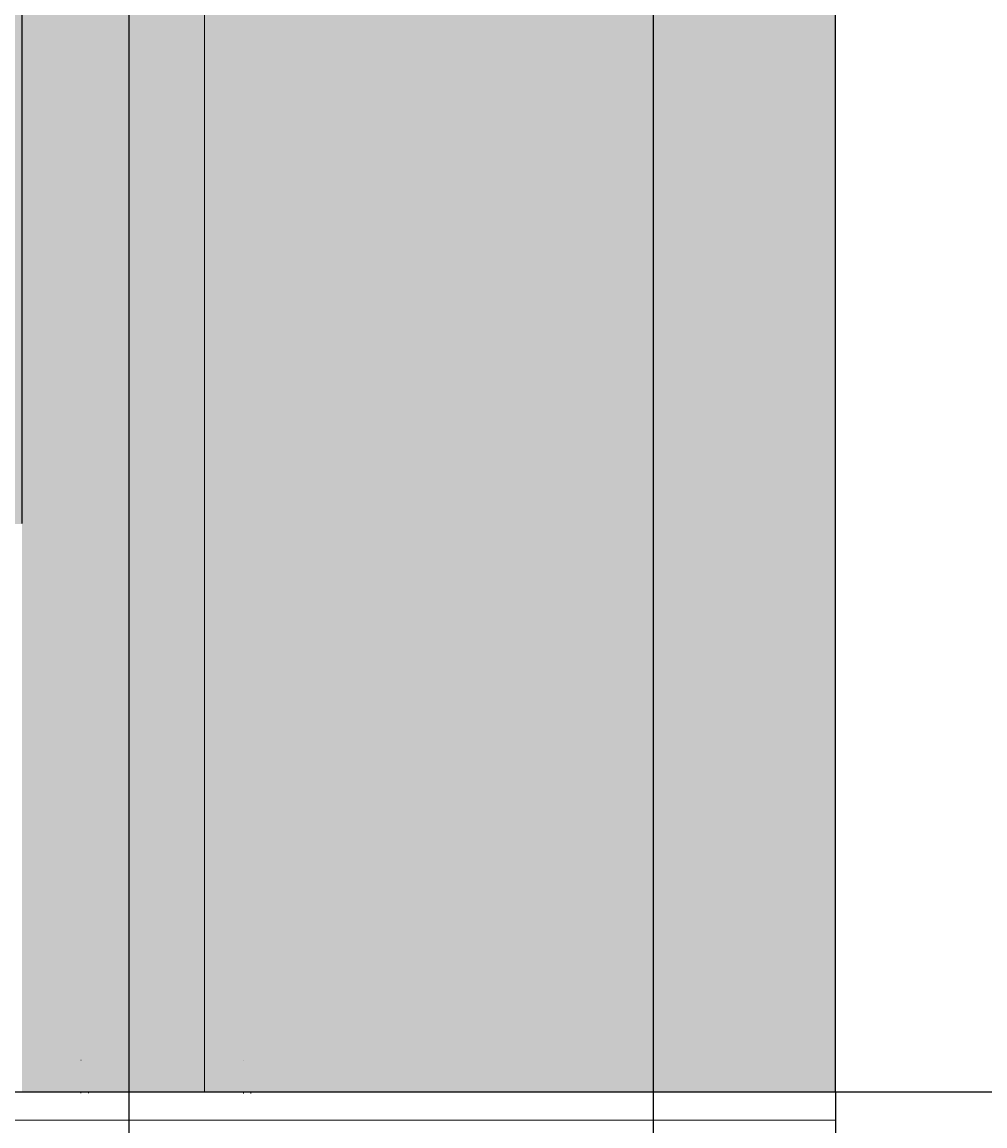
# Model space of a CAD drawing. Units: inches. Extents: x 36 to 594, y 79 to 831.
# Tile 25 of 30: x 342 to 468, y 446 to 590. Entities that reach past the tile are written whole.
import ezdxf

# ---------------------------------------------------------------- set-up
doc = ezdxf.new("R2010")
doc.units = ezdxf.units.IN
doc.header["$MEASUREMENT"] = 0
for name, color, linetype, lineweight in [('A-ANNO-DIMS', 2, 'Continuous', 18), ('A-ELEV', 7, 'Continuous', 25), ('A-ELEV-PATT', 8, 'Continuous', 13), ('A-GLAZ', 4, 'Continuous', 18)]:
    doc.layers.add(name, color=color, linetype=linetype, lineweight=lineweight)
doc.styles.get("Standard").update_dxf_attribs({"font": 'arial.ttf'})
doc.dimstyles.get("Standard").update_dxf_attribs({"dimtxt": 0.8125, "dimasz": 0.18, "dimexe": 0.18, "dimexo": 0.0625, "dimgap": 0.09, "dimtad": 0, "dimtih": 1, "dimtoh": 1, "dimdec": 4, "dimzin": 0, "dimdsep": 46, "dimlunit": 4, "dimtxsty": 'Standard', "dimcen": 0.09, "dimadec": 0, "dimazin": 0, "dimtfac": 1, "dimtdec": 4, "dimtofl": 0, "dimtmove": 0, "dimatfit": 3, "dimfxl": 1, "dimtolj": 1, "dimtzin": 0, "dimarcsym": 0})

# ---------------------------------------------------------------- blocks, each defined once
blk = doc.blocks.new('*D34')
at = {"layer": 'A-ANNO-DIMS', "color": 0, "lineweight": -2, "transparency": 16777216}
for p, q in [((448.45, 450.21), (592.85, 450.21)), ((592.67, 450.03), (592.67, 438.48)), ((592.67, 425.91), (592.67, 437.47)), ((424.61, 425.73), (592.85, 425.73))]:
    blk.add_line(p, q, dxfattribs=at)
at = {"layer": 'A-ANNO-DIMS', "color": 0, "transparency": 16777216}
for points in [[(592.64, 450.03), (592.7, 450.03), (592.67, 450.21)], [(592.64, 425.91), (592.7, 425.91), (592.67, 425.73)]]:
    blk.add_solid(points, dxfattribs=at)
at = {"layer": 'Defpoints', "color": 0, "transparency": 16777216}
for p in [(448.39, 450.21), (592.67, 450.21), (424.55, 425.73)]:
    blk.add_point(p, dxfattribs=at)
at = {"layer": 'A-ANNO-DIMS', "color": 0, "transparency": 16777216, "insert": (592.67, 437.97), "char_height": 0.812, "attachment_point": 5}
blk.add_mtext('\\A1;24.48', dxfattribs=at)
blk = doc.blocks.new('*D35')
at = {"layer": 'A-ANNO-DIMS', "color": 0, "lineweight": -2, "transparency": 16777216}
for p, q in [((424.56, 594.21), (592.85, 594.21)), ((592.67, 594.03), (592.67, 522.71)), ((592.67, 450.39), (592.67, 521.71)), ((448.45, 450.21), (592.85, 450.21))]:
    blk.add_line(p, q, dxfattribs=at)
at = {"layer": 'A-ANNO-DIMS', "color": 0, "transparency": 16777216}
for points in [[(592.64, 594.03), (592.7, 594.03), (592.67, 594.21)], [(592.64, 450.39), (592.7, 450.39), (592.67, 450.21)]]:
    blk.add_solid(points, dxfattribs=at)
at = {"layer": 'Defpoints', "color": 0, "transparency": 16777216}
for p in [(424.5, 594.21), (592.67, 594.21), (448.39, 450.21)]:
    blk.add_point(p, dxfattribs=at)
at = {"layer": 'A-ANNO-DIMS', "color": 0, "transparency": 16777216, "insert": (592.67, 522.21), "char_height": 0.812, "attachment_point": 5}
blk.add_mtext('\\A1;144', dxfattribs=at)
blk = doc.blocks.new('*D59')
at = {"layer": 'A-ANNO-DIMS', "color": 0, "lineweight": -2, "transparency": 16777216}
for p, q in [((355.86, 355.15), (355.86, 830.73)), ((356.04, 830.55), (388.74, 830.55)), ((424.37, 830.55), (391.67, 830.55)), ((424.55, 355.15), (424.55, 830.73))]:
    blk.add_line(p, q, dxfattribs=at)
at = {"layer": 'A-ANNO-DIMS', "color": 0, "transparency": 16777216}
for points in [[(356.04, 830.58), (356.04, 830.52), (355.86, 830.55)], [(424.37, 830.58), (424.37, 830.52), (424.55, 830.55)]]:
    blk.add_solid(points, dxfattribs=at)
at = {"layer": 'Defpoints', "color": 0, "transparency": 16777216}
for p in [(424.55, 830.55), (355.86, 355.08), (424.55, 355.08)]:
    blk.add_point(p, dxfattribs=at)
at = {"layer": 'A-ANNO-DIMS', "color": 0, "transparency": 16777216, "insert": (390.2, 830.55), "char_height": 0.812, "attachment_point": 5}
blk.add_mtext('\\A1;68.69', dxfattribs=at)
blk = doc.blocks.new('*D95')
at = {"layer": 'A-ANNO-DIMS', "color": 0, "lineweight": -2, "transparency": 16777216}
for p, q in [((260.51, 524.67), (260.51, 830.73)), ((260.69, 830.55), (299.71, 830.55)), ((341.66, 830.55), (302.63, 830.55)), ((341.84, 524.67), (341.84, 830.73))]:
    blk.add_line(p, q, dxfattribs=at)
at = {"layer": 'A-ANNO-DIMS', "color": 0, "transparency": 16777216}
for points in [[(260.69, 830.58), (260.69, 830.52), (260.51, 830.55)], [(341.66, 830.58), (341.66, 830.52), (341.84, 830.55)]]:
    blk.add_solid(points, dxfattribs=at)
at = {"layer": 'Defpoints', "color": 0, "transparency": 16777216}
for p in [(341.84, 830.55), (260.51, 524.6), (341.84, 524.6)]:
    blk.add_point(p, dxfattribs=at)
at = {"layer": 'A-ANNO-DIMS', "color": 0, "transparency": 16777216, "insert": (301.17, 830.55), "char_height": 0.812, "attachment_point": 5}
blk.add_mtext('\\A1;81.33', dxfattribs=at)
blk = doc.blocks.new('*D107')
at = {"layer": 'A-ANNO-DIMS', "color": 0, "lineweight": -2, "transparency": 16777216}
for p, q in [((269.04, 404.34), (269.04, 830.73)), ((269.22, 830.55), (310.99, 830.55)), ((355.68, 830.55), (313.91, 830.55)), ((355.86, 404.34), (355.86, 830.73))]:
    blk.add_line(p, q, dxfattribs=at)
at = {"layer": 'A-ANNO-DIMS', "color": 0, "transparency": 16777216}
for points in [[(269.22, 830.58), (269.22, 830.52), (269.04, 830.55)], [(355.68, 830.58), (355.68, 830.52), (355.86, 830.55)]]:
    blk.add_solid(points, dxfattribs=at)
at = {"layer": 'Defpoints', "color": 0, "transparency": 16777216}
for p in [(355.86, 830.55), (269.04, 404.27), (355.86, 404.27)]:
    blk.add_point(p, dxfattribs=at)
at = {"layer": 'A-ANNO-DIMS', "color": 0, "transparency": 16777216, "insert": (312.45, 830.55), "char_height": 0.812, "attachment_point": 5}
blk.add_mtext('\\A1;86.82', dxfattribs=at)

msp = doc.modelspace()

# ---------------------------------------------------------------- hatches: boundary and pattern name
at = {"layer": 'A-ELEV-PATT'}
h = msp.add_hatch(color=256, dxfattribs=at)
h.dxf.hatch_style = 1
h.paths.add_polyline_path([(398.0873, 796.0465), (269.3592, 796.0465), (269.3592, 770.1455), (397.8159, 770.1455)])
h.paths.add_polyline_path([(397.7518, 764.0341), (269.3592, 764.0341), (269.3592, 630.0394), (341.8367, 630.0394), (341.8367, 720.595), (335.0881, 728.3699), (329.982, 735.3373), (345.3661, 727.7743), (397.1052, 702.3389)])
h.paths.add_polyline_path([(341.8367, 594.2124), (201.4189, 594.2124), (201.4189, 475.4136), (232.8216, 475.4136), (232.8216, 524.6037), (341.8367, 524.6037)])
h.paths.add_polyline_path([(177.525, 594.2124), (118.7598, 594.2124), (118.7598, 450.2124), (177.525, 450.2124)])
h.paths.add_polyline_path([(424.4958, 594.2124), (365.7306, 594.2124), (365.7306, 450.2124), (424.4958, 450.2124)])
h.paths.add_polyline_path([(241.3553, 404.2737), (355.8569, 404.2737), (355.8569, 355.0836), (424.5492, 355.0836), (424.5492, 425.7333), (118.7598, 426.2844), (118.7598, 355.0836), (241.3553, 355.0836)])
h.paths.add_polyline_path([(448.3898, 306.2124), (217.0273, 306.2124), (217.0273, 142.2124), (254.0293, 142.2124), (254.0293, 150.9347), (254.0293, 286.1802), (401.5491, 286.1802), (401.5491, 150.9347), (401.5491, 142.2124), (448.3898, 142.2124)])
h.paths.add_polyline_path([(448.3898, 142.2124), (401.5491, 142.2124), (217.0273, 142.2124), (217.0273, 114.2124), (448.3898, 114.2124)])
h.paths.add_polyline_path([(217.0273, 306.2124), (174.7353, 306.2124), (94.8658, 306.2124), (94.8658, 162.2124), (103.3368, 162.2124), (103.3368, 264.6224), (103.3368, 286.1802), (217.0273, 286.1802)])
h = msp.add_hatch(color=256, dxfattribs=at)
h.dxf.hatch_style = 1
h.paths.add_polyline_path([(448.3898, 668.2124), (341.8367, 720.595), (341.8367, 594.2124), (341.8367, 450.2124), (365.7306, 450.2124), (365.7306, 594.2124), (424.4958, 594.2124), (424.4958, 450.2124), (448.3898, 450.2124), (448.3898, 594.2124)])
h.paths.add_polyline_path([(378.5958, 653.8563, -1), (413.2033, 653.8563, -1)], flags=16)
h.paths.add_polyline_path([(394.8995, 653.8563), (394.8995, 654.8563), (395.8995, 654.8563), (396.8995, 654.8563), (396.8995, 653.8563), (396.8995, 652.8563), (395.8995, 652.8563), (394.8995, 652.8563)], flags=0)
h.paths.add_polyline_path([(201.4189, 708.8485), (201.4189, 720.595), (94.8658, 668.2124), (94.8658, 644.2124), (94.8658, 596.2124), (94.8658, 594.2124), (94.8658, 450.2124), (118.7598, 450.2124), (118.7598, 594.2124), (177.525, 594.2124), (177.525, 450.2124), (201.4189, 450.2124), (201.4189, 594.2124)])
h.paths.add_polyline_path([(130.1589, 653.7648, -1), (164.7665, 653.7648, -1)], flags=16)
h.paths.add_polyline_path([(148.4627, 652.7648), (147.4627, 652.7648), (146.4627, 652.7648), (146.4627, 653.7648), (146.4627, 654.7648), (147.4627, 654.7648), (148.4627, 654.7648), (148.4627, 653.7648)], flags=0)
h = msp.add_hatch(dxfattribs=at)
h.set_pattern_fill('ANSI31', color=256, scale=38, angle=135)
h.paths.add_polyline_path([(448.3898, 450.2124), (94.8658, 450.2124), (94.8658, 306.2124), (174.7353, 306.2124), (448.3898, 306.2124), (448.3898, 367.5118)])
h.paths.add_polyline_path([(424.5492, 425.7333), (424.5492, 329.5325), (118.7598, 330.0836), (118.7598, 354.0836), (118.7598, 426.2844)], flags=16)
h.paths.add_polyline_path([(355.8569, 404.2737), (355.8569, 355.0836), (241.3553, 355.0836), (241.3553, 404.2737)], flags=0)
h.paths.add_polyline_path([(269.0393, 390.7924), (269.0393, 355.0836), (244.8248, 355.0836), (244.8248, 364.0887), (263.8892, 364.0887), (263.8892, 355.0836), (267.0393, 355.0836), (267.0393, 390.7924)], flags=0)
h.paths.add_polyline_path([(303.9765, 436.9126, -1), (313.1496, 436.9126, -1)], flags=16)
h.paths.add_polyline_path([(421.9473, 354.0836), (421.9376, 348.6883), (421.9376, 333.9204), (401.6342, 333.9204), (401.6705, 354.0836), (400.6705, 354.0836), (400.6608, 348.7267), (400.6608, 333.9587), (380.3574, 333.9587), (380.3937, 354.0836), (379.3937, 354.0836), (379.3841, 348.765), (379.3841, 333.997), (359.0807, 333.997), (359.1169, 354.0836), (358.1169, 354.0836), (358.1074, 348.8034), (358.1074, 334.0354), (337.804, 334.0354), (337.8401, 354.0836), (336.8401, 354.0836), (336.8306, 348.8417), (336.8306, 334.0737), (316.5272, 334.0737), (316.5633, 354.0836), (315.5633, 354.0836), (315.5539, 348.8801), (315.5539, 334.1121), (295.2505, 334.1121), (295.2865, 354.0836), (294.2865, 354.0836), (294.2772, 348.9184), (294.2772, 334.1504), (273.9738, 334.1504), (274.0097, 354.0836), (273.0097, 354.0836), (273.0005, 348.9568), (273.0005, 334.1888), (252.697, 334.1888), (252.7329, 354.0836), (251.7329, 354.0836), (251.7237, 348.9951), (251.7237, 334.2271), (231.4203, 334.2271), (231.4561, 354.0836), (230.4561, 354.0836), (230.447, 349.0335), (230.447, 334.2655), (210.1436, 334.2655), (210.1793, 354.0836), (209.1793, 354.0836), (209.1703, 349.0718), (209.1703, 334.3038), (188.8668, 334.3038), (188.9025, 354.0836), (187.9025, 354.0836), (187.8935, 349.1101), (187.8935, 334.3422), (167.5901, 334.3422), (167.6257, 354.0836), (166.6257, 354.0836), (166.6168, 349.1485), (166.6168, 334.3805), (146.3134, 334.3805), (146.3489, 354.0836), (145.3489, 354.0836), (145.3401, 349.1868), (145.3401, 334.4189), (125.0366, 334.4189), (125.0721, 354.0836)], flags=0)
h.paths.add_polyline_path([(266.285, 436.9126, -1), (275.458, 436.9126, -1)], flags=16)
h.paths.add_polyline_path([(367.0204, 316.8739, -1), (357.8474, 316.8739, -1)], flags=16)
h.paths.add_polyline_path([(347.6933, 316.8739, -1), (338.5202, 316.8739, -1)], flags=16)
h.paths.add_polyline_path([(329.574, 316.8739, -1), (320.401, 316.8739, -1)], flags=16)
h.paths.add_polyline_path([(263.8892, 385.1199), (263.8892, 368.1628), (244.8248, 368.1628), (244.8248, 385.1199)], flags=0)
h.paths.add_polyline_path([(216.2543, 436.9126, -1), (225.4274, 436.9126, -1)], flags=16)
h.paths.add_polyline_path([(275.458, 316.8739, -1), (266.285, 316.8739, -1)], flags=16)
h.paths.add_polyline_path([(225.4274, 316.8739, -1), (216.2543, 316.8739, -1)], flags=16)

# ---------------------------------------------------------------- linework, layer by layer
at = {"layer": 'A-ELEV'}
for p, q in [((448.3898, 450.2124), (448.3898, 594.2124)), ((94.8658, 450.2124), (448.3898, 450.2124)), ((448.3898, 450.2124), (448.3898, 367.5118))]:
    msp.add_line(p, q, dxfattribs=at)
at = {"layer": 'A-GLAZ'}
for p, q in [((365.7306, 450.2124), (365.7306, 594.2124)), ((424.4958, 450.2124), (424.4958, 594.2124)), ((349.5396, 450.2124), (349.5392, 450.0206)), ((350.5396, 450.2124), (350.5392, 450.0188)), ((370.8164, 450.2124), (370.8159, 449.9823)), ((371.8164, 450.2124), (371.8159, 449.9805))]:
    msp.add_line(p, q, dxfattribs=at)
for points in [[(349.5737, 454.3654), (349.547, 454.3654)], [(370.8504, 454.3271), (370.8238, 454.3271)]]:
    msp.add_lwpolyline(points, dxfattribs=at)

# ---------------------------------------------------------------- dimensions: what is measured, and where the dimension line sits
at = {"layer": 'A-ANNO-DIMS'}
for base, p1, p2, picture, middle in [((341.8367, 830.5465), (260.5056, 524.6037), (341.8367, 524.6037), '*D95', (301.1711, 830.5465)), ((355.8569, 830.5465), (269.0393, 404.2737), (355.8569, 404.2737), '*D107', (312.4481, 830.5465)), ((424.5492, 830.5465), (355.8569, 355.0836), (424.5492, 355.0836), '*D59', (390.203, 830.5465))]:
    dim = msp.add_linear_dim(base=base, p1=p1, p2=p2, dimstyle='Standard', override={"dimdec": 2, "dimlfac": 1, "dimrnd": 0, "dimzin": 0, "dimdsep": 46, "dimlunit": 2}, dxfattribs=at)
    dim.commit()
    dim.dimension.update_dxf_attribs({"geometry": picture, "text_midpoint": middle})
for base, p1, p2, override, picture, middle in [((592.6689, 594.2124), (448.3898, 450.2124), (424.4958, 594.2124), {"dimdec": 0, "dimlfac": 1, "dimrnd": 0, "dimzin": 0, "dimdsep": 46, "dimlunit": 2}, '*D35', (592.6689, 522.2124)), ((592.6689, 450.2124), (424.5492, 425.7333), (448.3898, 450.2124), {"dimdec": 2, "dimlfac": 1, "dimrnd": 0, "dimzin": 0, "dimdsep": 46, "dimlunit": 2}, '*D34', (592.6689, 437.9728))]:
    dim = msp.add_linear_dim(base=base, p1=p1, p2=p2, angle=90, dimstyle='Standard', override=override, dxfattribs=at)
    dim.commit()
    dim.dimension.update_dxf_attribs({"geometry": picture, "text_midpoint": middle})

doc.saveas('drawing.dxf')
